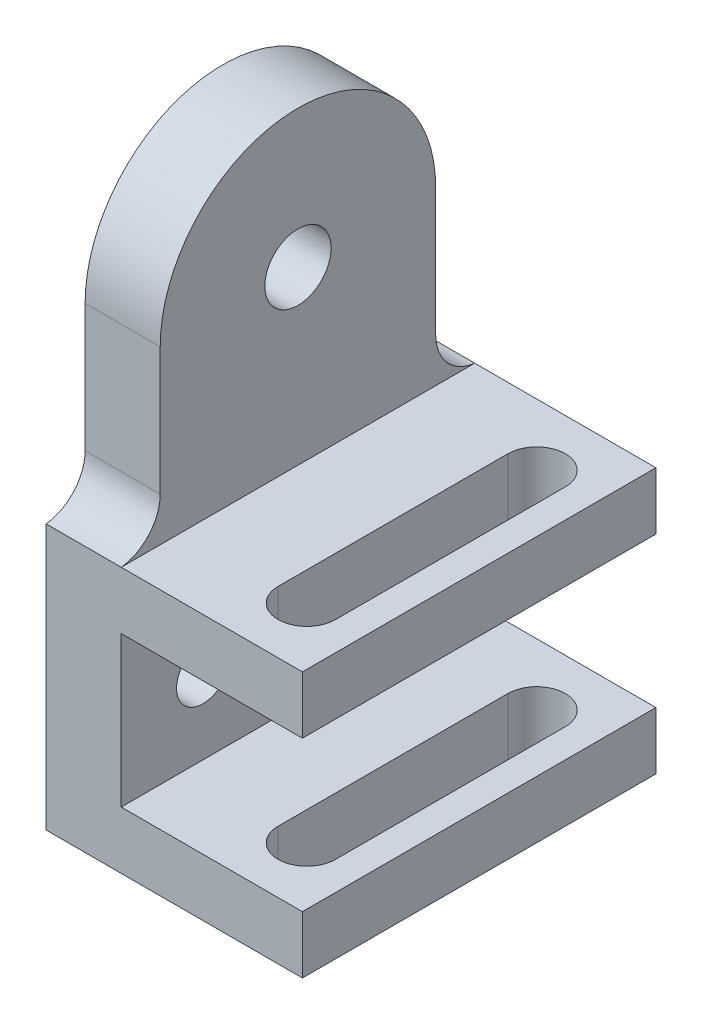
ISO-10303-21;
HEADER;
FILE_DESCRIPTION(('STEP AP214'),'2;1');
FILE_NAME('part.step','',(''),(''),'','','');
FILE_SCHEMA(('AUTOMOTIVE_DESIGN { 1 0 10303 214 1 1 1 1 }'));
ENDSEC;
DATA;
#1=APPLICATION_CONTEXT('core data for automotive mechanical design processes');
#2=APPLICATION_PROTOCOL_DEFINITION('international standard','automotive_design',2000,#1);
#3=PRODUCT_CONTEXT('',#1,'mechanical');
#4=PRODUCT('Part','Part','',(#3));
#5=PRODUCT_RELATED_PRODUCT_CATEGORY('part','',(#4));
#6=PRODUCT_DEFINITION_FORMATION('','',#4);
#7=PRODUCT_DEFINITION_CONTEXT('part definition',#1,'design');
#8=PRODUCT_DEFINITION('design','',#6,#7);
#9=PRODUCT_DEFINITION_SHAPE('','',#8);
#10=(LENGTH_UNIT() NAMED_UNIT(*) SI_UNIT(.MILLI.,.METRE.));
#11=(NAMED_UNIT(*) PLANE_ANGLE_UNIT() SI_UNIT($,.RADIAN.));
#12=(NAMED_UNIT(*) SI_UNIT($,.STERADIAN.) SOLID_ANGLE_UNIT());
#13=UNCERTAINTY_MEASURE_WITH_UNIT(LENGTH_MEASURE(1.E-05),#10,'distance_accuracy_value','');
#14=(GEOMETRIC_REPRESENTATION_CONTEXT(3) GLOBAL_UNCERTAINTY_ASSIGNED_CONTEXT((#13)) GLOBAL_UNIT_ASSIGNED_CONTEXT((#10,
#11,#12)) REPRESENTATION_CONTEXT('',''));
#15=CARTESIAN_POINT('',(0.,0.,0.));
#16=DIRECTION('',(0.,0.,1.));
#17=DIRECTION('',(1.,0.,0.));
#18=AXIS2_PLACEMENT_3D('',#15,#16,#17);
#19=CARTESIAN_POINT('',(0.,0.,40.));
#20=DIRECTION('',(1.,0.,0.));
#21=DIRECTION('',(0.,0.,-1.));
#22=AXIS2_PLACEMENT_3D('',#19,#20,#21);
#23=PLANE('',#22);
#24=CARTESIAN_POINT('',(0.,30.,-21.5));
#25=DIRECTION('',(1.,0.,0.));
#26=DIRECTION('',(0.,0.,-1.));
#27=AXIS2_PLACEMENT_3D('',#24,#25,#26);
#28=CIRCLE('',#27,6.);
#29=CARTESIAN_POINT('',(0.,30.,-27.5));
#30=VERTEX_POINT('',#29);
#31=EDGE_CURVE('E259',#30,#30,#28,.T.);
#32=ORIENTED_EDGE('',*,*,#31,.T.);
#33=EDGE_LOOP('',(#32));
#34=FACE_BOUND('',#33,.T.);
#35=CARTESIAN_POINT('',(0.,30.,21.5));
#36=DIRECTION('',(1.,0.,0.));
#37=DIRECTION('',(0.,0.,-1.));
#38=AXIS2_PLACEMENT_3D('',#35,#36,#37);
#39=CIRCLE('',#38,6.);
#40=CARTESIAN_POINT('',(0.,30.,15.5));
#41=VERTEX_POINT('',#40);
#42=EDGE_CURVE('E255',#41,#41,#39,.T.);
#43=ORIENTED_EDGE('',*,*,#42,.T.);
#44=EDGE_LOOP('',(#43));
#45=FACE_BOUND('',#44,.T.);
#46=CARTESIAN_POINT('',(0.,98.8253035818014,0.));
#47=DIRECTION('',(1.,0.,0.));
#48=DIRECTION('',(0.,0.,-1.));
#49=AXIS2_PLACEMENT_3D('',#46,#47,#48);
#50=CIRCLE('',#49,7.5);
#51=CARTESIAN_POINT('',(0.,98.8253035818014,-7.5));
#52=VERTEX_POINT('',#51);
#53=EDGE_CURVE('E264',#52,#52,#50,.T.);
#54=ORIENTED_EDGE('',*,*,#53,.T.);
#55=EDGE_LOOP('',(#54));
#56=FACE_BOUND('',#55,.T.);
#57=DIRECTION('',(0.,-1.,0.));
#58=VECTOR('',#57,1.);
#59=CARTESIAN_POINT('',(0.,0.,31.1746964181986));
#60=LINE('',#59,#58);
#61=CARTESIAN_POINT('',(0.,98.8253035818014,31.1746964181986));
#62=VERTEX_POINT('',#61);
#63=CARTESIAN_POINT('',(0.,69.9307647401936,31.1746964181986));
#64=VERTEX_POINT('',#63);
#65=EDGE_CURVE('E285',#62,#64,#60,.T.);
#66=ORIENTED_EDGE('',*,*,#65,.F.);
#67=CARTESIAN_POINT('',(0.,98.8253035818014,0.));
#68=DIRECTION('',(1.,0.,0.));
#69=DIRECTION('',(0.,0.,-1.));
#70=AXIS2_PLACEMENT_3D('',#67,#68,#69);
#71=CIRCLE('',#70,31.1746964181986);
#72=CARTESIAN_POINT('',(0.,98.8253035818014,-31.1746964181986));
#73=VERTEX_POINT('',#72);
#74=EDGE_CURVE('E297',#73,#62,#71,.T.);
#75=ORIENTED_EDGE('',*,*,#74,.F.);
#76=DIRECTION('',(0.,1.,0.));
#77=VECTOR('',#76,1.);
#78=CARTESIAN_POINT('',(0.,0.,-31.1746964181986));
#79=LINE('',#78,#77);
#80=CARTESIAN_POINT('',(0.,69.9307647401936,-31.1746964181986));
#81=VERTEX_POINT('',#80);
#82=EDGE_CURVE('E299',#81,#73,#79,.T.);
#83=ORIENTED_EDGE('',*,*,#82,.F.);
#84=CARTESIAN_POINT('',(0.,69.9307647401936,-41.1746964181986));
#85=DIRECTION('',(1.,0.,0.));
#86=DIRECTION('',(0.,0.,-1.));
#87=AXIS2_PLACEMENT_3D('',#84,#85,#86);
#88=CIRCLE('',#87,10.);
#89=CARTESIAN_POINT('',(0.,60.,-40.));
#90=VERTEX_POINT('',#89);
#91=EDGE_CURVE('E293',#90,#81,#88,.F.);
#92=ORIENTED_EDGE('',*,*,#91,.F.);
#93=DIRECTION('',(0.,-1.,0.));
#94=VECTOR('',#93,1.);
#95=CARTESIAN_POINT('',(0.,0.,-40.));
#96=LINE('',#95,#94);
#97=CARTESIAN_POINT('',(0.,0.,-40.));
#98=VERTEX_POINT('',#97);
#99=EDGE_CURVE('E304',#90,#98,#96,.T.);
#100=ORIENTED_EDGE('',*,*,#99,.T.);
#101=DIRECTION('',(0.,0.,-1.));
#102=VECTOR('',#101,1.);
#103=CARTESIAN_POINT('',(0.,0.,40.));
#104=LINE('',#103,#102);
#105=CARTESIAN_POINT('',(0.,0.,40.));
#106=VERTEX_POINT('',#105);
#107=EDGE_CURVE('E359',#106,#98,#104,.T.);
#108=ORIENTED_EDGE('',*,*,#107,.F.);
#109=DIRECTION('',(0.,-1.,0.));
#110=VECTOR('',#109,1.);
#111=CARTESIAN_POINT('',(0.,0.,40.));
#112=LINE('',#111,#110);
#113=CARTESIAN_POINT('',(0.,60.,40.));
#114=VERTEX_POINT('',#113);
#115=EDGE_CURVE('E305',#114,#106,#112,.T.);
#116=ORIENTED_EDGE('',*,*,#115,.F.);
#117=CARTESIAN_POINT('',(0.,69.9307647401936,41.1746964181986));
#118=DIRECTION('',(1.,0.,0.));
#119=DIRECTION('',(0.,0.,-1.));
#120=AXIS2_PLACEMENT_3D('',#117,#118,#119);
#121=CIRCLE('',#120,10.);
#122=EDGE_CURVE('E279',#114,#64,#121,.T.);
#123=ORIENTED_EDGE('',*,*,#122,.T.);
#124=EDGE_LOOP('',(#66,#75,#83,#92,#100,#108,#116,#123));
#125=FACE_BOUND('',#124,.T.);
#126=ADVANCED_FACE('F39',(#34,#45,#56,#125),#23,.F.);
#127=CARTESIAN_POINT('',(17.,60.,40.));
#128=DIRECTION('',(-1.,0.,0.));
#129=DIRECTION('',(0.,0.,1.));
#130=AXIS2_PLACEMENT_3D('',#127,#128,#129);
#131=PLANE('',#130);
#132=CARTESIAN_POINT('',(17.,98.8253035818014,0.));
#133=DIRECTION('',(1.,0.,0.));
#134=DIRECTION('',(0.,0.,-1.));
#135=AXIS2_PLACEMENT_3D('',#132,#133,#134);
#136=CIRCLE('',#135,7.5);
#137=CARTESIAN_POINT('',(17.,98.8253035818014,-7.5));
#138=VERTEX_POINT('',#137);
#139=EDGE_CURVE('E265',#138,#138,#136,.T.);
#140=ORIENTED_EDGE('',*,*,#139,.F.);
#141=EDGE_LOOP('',(#140));
#142=FACE_BOUND('',#141,.T.);
#143=CARTESIAN_POINT('',(17.,98.8253035818014,0.));
#144=DIRECTION('',(1.,0.,0.));
#145=DIRECTION('',(0.,0.,-1.));
#146=AXIS2_PLACEMENT_3D('',#143,#144,#145);
#147=CIRCLE('',#146,31.1746964181986);
#148=CARTESIAN_POINT('',(17.,98.8253035818014,-31.1746964181986));
#149=VERTEX_POINT('',#148);
#150=CARTESIAN_POINT('',(17.,98.8253035818014,31.1746964181986));
#151=VERTEX_POINT('',#150);
#152=EDGE_CURVE('E289',#149,#151,#147,.T.);
#153=ORIENTED_EDGE('',*,*,#152,.T.);
#154=DIRECTION('',(0.,-1.,0.));
#155=VECTOR('',#154,1.);
#156=CARTESIAN_POINT('',(17.,0.,31.1746964181986));
#157=LINE('',#156,#155);
#158=CARTESIAN_POINT('',(17.,69.9307647401936,31.1746964181986));
#159=VERTEX_POINT('',#158);
#160=EDGE_CURVE('E271',#151,#159,#157,.T.);
#161=ORIENTED_EDGE('',*,*,#160,.T.);
#162=CARTESIAN_POINT('',(17.,69.9307647401936,41.1746964181986));
#163=DIRECTION('',(1.,0.,0.));
#164=DIRECTION('',(0.,0.,-1.));
#165=AXIS2_PLACEMENT_3D('',#162,#163,#164);
#166=CIRCLE('',#165,10.);
#167=CARTESIAN_POINT('',(17.,60.,40.));
#168=VERTEX_POINT('',#167);
#169=EDGE_CURVE('E268',#168,#159,#166,.T.);
#170=ORIENTED_EDGE('',*,*,#169,.F.);
#171=DIRECTION('',(0.,0.,-1.));
#172=VECTOR('',#171,1.);
#173=CARTESIAN_POINT('',(17.,60.,40.));
#174=LINE('',#173,#172);
#175=CARTESIAN_POINT('',(17.,60.,-40.));
#176=VERTEX_POINT('',#175);
#177=EDGE_CURVE('E321',#168,#176,#174,.T.);
#178=ORIENTED_EDGE('',*,*,#177,.T.);
#179=CARTESIAN_POINT('',(17.,69.9307647401936,-41.1746964181986));
#180=DIRECTION('',(1.,0.,0.));
#181=DIRECTION('',(0.,0.,-1.));
#182=AXIS2_PLACEMENT_3D('',#179,#180,#181);
#183=CIRCLE('',#182,10.);
#184=CARTESIAN_POINT('',(17.,69.9307647401936,-31.1746964181986));
#185=VERTEX_POINT('',#184);
#186=EDGE_CURVE('E283',#176,#185,#183,.F.);
#187=ORIENTED_EDGE('',*,*,#186,.T.);
#188=DIRECTION('',(0.,1.,0.));
#189=VECTOR('',#188,1.);
#190=CARTESIAN_POINT('',(17.,0.,-31.1746964181986));
#191=LINE('',#190,#189);
#192=EDGE_CURVE('E286',#185,#149,#191,.T.);
#193=ORIENTED_EDGE('',*,*,#192,.T.);
#194=EDGE_LOOP('',(#153,#161,#170,#178,#187,#193));
#195=FACE_BOUND('',#194,.T.);
#196=ADVANCED_FACE('F373',(#142,#195),#131,.F.);
#197=CARTESIAN_POINT('',(0.,0.,-40.));
#198=DIRECTION('',(0.,0.,-1.));
#199=DIRECTION('',(-1.,0.,0.));
#200=AXIS2_PLACEMENT_3D('',#197,#198,#199);
#201=PLANE('',#200);
#202=ORIENTED_EDGE('',*,*,#99,.F.);
#203=DIRECTION('',(1.,0.,0.));
#204=VECTOR('',#203,1.);
#205=CARTESIAN_POINT('',(-63.,60.,-40.));
#206=LINE('',#205,#204);
#207=EDGE_CURVE('E46',#90,#176,#206,.T.);
#208=ORIENTED_EDGE('',*,*,#207,.T.);
#209=DIRECTION('',(-1.,0.,0.));
#210=VECTOR('',#209,1.);
#211=CARTESIAN_POINT('',(58.,60.,-40.));
#212=LINE('',#211,#210);
#213=CARTESIAN_POINT('',(58.,60.,-40.));
#214=VERTEX_POINT('',#213);
#215=EDGE_CURVE('E308',#214,#176,#212,.T.);
#216=ORIENTED_EDGE('',*,*,#215,.F.);
#217=DIRECTION('',(0.,1.,0.));
#218=VECTOR('',#217,1.);
#219=CARTESIAN_POINT('',(58.,47.,-40.));
#220=LINE('',#219,#218);
#221=CARTESIAN_POINT('',(58.,47.,-40.));
#222=VERTEX_POINT('',#221);
#223=EDGE_CURVE('E334',#222,#214,#220,.T.);
#224=ORIENTED_EDGE('',*,*,#223,.F.);
#225=DIRECTION('',(1.,0.,0.));
#226=VECTOR('',#225,1.);
#227=CARTESIAN_POINT('',(17.,47.,-40.));
#228=LINE('',#227,#226);
#229=CARTESIAN_POINT('',(17.,47.,-40.));
#230=VERTEX_POINT('',#229);
#231=EDGE_CURVE('E332',#230,#222,#228,.T.);
#232=ORIENTED_EDGE('',*,*,#231,.F.);
#233=DIRECTION('',(0.,1.,0.));
#234=VECTOR('',#233,1.);
#235=CARTESIAN_POINT('',(17.,13.,-40.));
#236=LINE('',#235,#234);
#237=CARTESIAN_POINT('',(17.,13.,-40.));
#238=VERTEX_POINT('',#237);
#239=EDGE_CURVE('E328',#238,#230,#236,.T.);
#240=ORIENTED_EDGE('',*,*,#239,.F.);
#241=DIRECTION('',(-1.,0.,0.));
#242=VECTOR('',#241,1.);
#243=CARTESIAN_POINT('',(58.,13.,-40.));
#244=LINE('',#243,#242);
#245=CARTESIAN_POINT('',(58.,13.,-40.));
#246=VERTEX_POINT('',#245);
#247=EDGE_CURVE('E330',#246,#238,#244,.T.);
#248=ORIENTED_EDGE('',*,*,#247,.F.);
#249=DIRECTION('',(0.,1.,0.));
#250=VECTOR('',#249,1.);
#251=CARTESIAN_POINT('',(58.,0.,-40.));
#252=LINE('',#251,#250);
#253=CARTESIAN_POINT('',(58.,0.,-40.));
#254=VERTEX_POINT('',#253);
#255=EDGE_CURVE('E324',#254,#246,#252,.T.);
#256=ORIENTED_EDGE('',*,*,#255,.F.);
#257=DIRECTION('',(1.,0.,0.));
#258=VECTOR('',#257,1.);
#259=CARTESIAN_POINT('',(0.,0.,-40.));
#260=LINE('',#259,#258);
#261=EDGE_CURVE('E323',#98,#254,#260,.T.);
#262=ORIENTED_EDGE('',*,*,#261,.F.);
#263=EDGE_LOOP('',(#202,#208,#216,#224,#232,#240,#248,#256,#262));
#264=FACE_BOUND('',#263,.T.);
#265=ADVANCED_FACE('F361',(#264),#201,.T.);
#266=CARTESIAN_POINT('',(0.,0.,40.));
#267=DIRECTION('',(0.,1.,0.));
#268=DIRECTION('',(0.,0.,1.));
#269=AXIS2_PLACEMENT_3D('',#266,#267,#268);
#270=PLANE('',#269);
#271=DIRECTION('',(0.,0.,1.));
#272=VECTOR('',#271,1.);
#273=CARTESIAN_POINT('',(38.5,0.,40.));
#274=LINE('',#273,#272);
#275=CARTESIAN_POINT('',(38.5,0.,-26.));
#276=VERTEX_POINT('',#275);
#277=CARTESIAN_POINT('',(38.5,0.,26.));
#278=VERTEX_POINT('',#277);
#279=EDGE_CURVE('E236',#276,#278,#274,.T.);
#280=ORIENTED_EDGE('',*,*,#279,.T.);
#281=CARTESIAN_POINT('',(45.,0.,26.));
#282=DIRECTION('',(0.,1.,0.));
#283=DIRECTION('',(0.,0.,1.));
#284=AXIS2_PLACEMENT_3D('',#281,#282,#283);
#285=CIRCLE('',#284,6.5);
#286=CARTESIAN_POINT('',(51.5,0.,26.));
#287=VERTEX_POINT('',#286);
#288=EDGE_CURVE('E249',#278,#287,#285,.T.);
#289=ORIENTED_EDGE('',*,*,#288,.T.);
#290=DIRECTION('',(0.,0.,-1.));
#291=VECTOR('',#290,1.);
#292=CARTESIAN_POINT('',(51.5,0.,40.));
#293=LINE('',#292,#291);
#294=CARTESIAN_POINT('',(51.5,0.,-26.));
#295=VERTEX_POINT('',#294);
#296=EDGE_CURVE('E225',#287,#295,#293,.T.);
#297=ORIENTED_EDGE('',*,*,#296,.T.);
#298=CARTESIAN_POINT('',(45.,0.,-26.));
#299=DIRECTION('',(0.,1.,0.));
#300=DIRECTION('',(0.,0.,1.));
#301=AXIS2_PLACEMENT_3D('',#298,#299,#300);
#302=CIRCLE('',#301,6.5);
#303=EDGE_CURVE('E228',#295,#276,#302,.T.);
#304=ORIENTED_EDGE('',*,*,#303,.T.);
#305=EDGE_LOOP('',(#280,#289,#297,#304));
#306=FACE_BOUND('',#305,.T.);
#307=ORIENTED_EDGE('',*,*,#261,.T.);
#308=DIRECTION('',(0.,0.,-1.));
#309=VECTOR('',#308,1.);
#310=CARTESIAN_POINT('',(58.,0.,40.));
#311=LINE('',#310,#309);
#312=CARTESIAN_POINT('',(58.,0.,40.));
#313=VERTEX_POINT('',#312);
#314=EDGE_CURVE('E353',#313,#254,#311,.T.);
#315=ORIENTED_EDGE('',*,*,#314,.F.);
#316=DIRECTION('',(1.,0.,0.));
#317=VECTOR('',#316,1.);
#318=CARTESIAN_POINT('',(0.,0.,40.));
#319=LINE('',#318,#317);
#320=EDGE_CURVE('E303',#106,#313,#319,.T.);
#321=ORIENTED_EDGE('',*,*,#320,.F.);
#322=ORIENTED_EDGE('',*,*,#107,.T.);
#323=EDGE_LOOP('',(#307,#315,#321,#322));
#324=FACE_BOUND('',#323,.T.);
#325=ADVANCED_FACE('F406',(#306,#324),#270,.F.);
#326=CARTESIAN_POINT('',(58.,0.,40.));
#327=DIRECTION('',(-1.,0.,0.));
#328=DIRECTION('',(0.,0.,1.));
#329=AXIS2_PLACEMENT_3D('',#326,#327,#328);
#330=PLANE('',#329);
#331=ORIENTED_EDGE('',*,*,#255,.T.);
#332=DIRECTION('',(0.,0.,-1.));
#333=VECTOR('',#332,1.);
#334=CARTESIAN_POINT('',(58.,13.,40.));
#335=LINE('',#334,#333);
#336=CARTESIAN_POINT('',(58.,13.,40.));
#337=VERTEX_POINT('',#336);
#338=EDGE_CURVE('E351',#337,#246,#335,.T.);
#339=ORIENTED_EDGE('',*,*,#338,.F.);
#340=DIRECTION('',(0.,1.,0.));
#341=VECTOR('',#340,1.);
#342=CARTESIAN_POINT('',(58.,0.,40.));
#343=LINE('',#342,#341);
#344=EDGE_CURVE('E306',#313,#337,#343,.T.);
#345=ORIENTED_EDGE('',*,*,#344,.F.);
#346=ORIENTED_EDGE('',*,*,#314,.T.);
#347=EDGE_LOOP('',(#331,#339,#345,#346));
#348=FACE_BOUND('',#347,.T.);
#349=ADVANCED_FACE('F402',(#348),#330,.F.);
#350=CARTESIAN_POINT('',(58.,13.,40.));
#351=DIRECTION('',(0.,-1.,0.));
#352=DIRECTION('',(0.,0.,-1.));
#353=AXIS2_PLACEMENT_3D('',#350,#351,#352);
#354=PLANE('',#353);
#355=DIRECTION('',(0.,0.,1.));
#356=VECTOR('',#355,1.);
#357=CARTESIAN_POINT('',(51.5,13.,40.));
#358=LINE('',#357,#356);
#359=CARTESIAN_POINT('',(51.5,13.,-26.));
#360=VERTEX_POINT('',#359);
#361=CARTESIAN_POINT('',(51.5,13.,26.));
#362=VERTEX_POINT('',#361);
#363=EDGE_CURVE('E218',#360,#362,#358,.T.);
#364=ORIENTED_EDGE('',*,*,#363,.T.);
#365=CARTESIAN_POINT('',(45.,13.,26.));
#366=DIRECTION('',(0.,-1.,0.));
#367=DIRECTION('',(0.,0.,-1.));
#368=AXIS2_PLACEMENT_3D('',#365,#366,#367);
#369=CIRCLE('',#368,6.5);
#370=CARTESIAN_POINT('',(38.5,13.,26.));
#371=VERTEX_POINT('',#370);
#372=EDGE_CURVE('E243',#362,#371,#369,.T.);
#373=ORIENTED_EDGE('',*,*,#372,.T.);
#374=DIRECTION('',(0.,0.,-1.));
#375=VECTOR('',#374,1.);
#376=CARTESIAN_POINT('',(38.5,13.,40.));
#377=LINE('',#376,#375);
#378=CARTESIAN_POINT('',(38.5,13.,-26.));
#379=VERTEX_POINT('',#378);
#380=EDGE_CURVE('E233',#371,#379,#377,.T.);
#381=ORIENTED_EDGE('',*,*,#380,.T.);
#382=CARTESIAN_POINT('',(45.,13.,-26.));
#383=DIRECTION('',(0.,-1.,0.));
#384=DIRECTION('',(0.,0.,-1.));
#385=AXIS2_PLACEMENT_3D('',#382,#383,#384);
#386=CIRCLE('',#385,6.5);
#387=EDGE_CURVE('E226',#379,#360,#386,.T.);
#388=ORIENTED_EDGE('',*,*,#387,.T.);
#389=EDGE_LOOP('',(#364,#373,#381,#388));
#390=FACE_BOUND('',#389,.T.);
#391=ORIENTED_EDGE('',*,*,#247,.T.);
#392=DIRECTION('',(0.,0.,-1.));
#393=VECTOR('',#392,1.);
#394=CARTESIAN_POINT('',(17.,13.,40.));
#395=LINE('',#394,#393);
#396=CARTESIAN_POINT('',(17.,13.,40.));
#397=VERTEX_POINT('',#396);
#398=EDGE_CURVE('E346',#397,#238,#395,.T.);
#399=ORIENTED_EDGE('',*,*,#398,.F.);
#400=DIRECTION('',(-1.,0.,0.));
#401=VECTOR('',#400,1.);
#402=CARTESIAN_POINT('',(58.,13.,40.));
#403=LINE('',#402,#401);
#404=EDGE_CURVE('E309',#337,#397,#403,.T.);
#405=ORIENTED_EDGE('',*,*,#404,.F.);
#406=ORIENTED_EDGE('',*,*,#338,.T.);
#407=EDGE_LOOP('',(#391,#399,#405,#406));
#408=FACE_BOUND('',#407,.T.);
#409=ADVANCED_FACE('F399',(#390,#408),#354,.F.);
#410=CARTESIAN_POINT('',(17.,13.,40.));
#411=DIRECTION('',(-1.,0.,0.));
#412=DIRECTION('',(0.,0.,1.));
#413=AXIS2_PLACEMENT_3D('',#410,#411,#412);
#414=PLANE('',#413);
#415=CARTESIAN_POINT('',(17.,30.,-21.5));
#416=DIRECTION('',(1.,0.,0.));
#417=DIRECTION('',(0.,0.,1.));
#418=AXIS2_PLACEMENT_3D('',#415,#416,#417);
#419=CIRCLE('',#418,6.);
#420=CARTESIAN_POINT('',(17.,30.,-15.5));
#421=VERTEX_POINT('',#420);
#422=EDGE_CURVE('E253',#421,#421,#419,.T.);
#423=ORIENTED_EDGE('',*,*,#422,.F.);
#424=EDGE_LOOP('',(#423));
#425=FACE_BOUND('',#424,.T.);
#426=CARTESIAN_POINT('',(17.,30.,21.5));
#427=DIRECTION('',(1.,0.,0.));
#428=DIRECTION('',(0.,0.,-1.));
#429=AXIS2_PLACEMENT_3D('',#426,#427,#428);
#430=CIRCLE('',#429,6.);
#431=CARTESIAN_POINT('',(17.,30.,15.5));
#432=VERTEX_POINT('',#431);
#433=EDGE_CURVE('E248',#432,#432,#430,.T.);
#434=ORIENTED_EDGE('',*,*,#433,.F.);
#435=EDGE_LOOP('',(#434));
#436=FACE_BOUND('',#435,.T.);
#437=ORIENTED_EDGE('',*,*,#239,.T.);
#438=DIRECTION('',(0.,0.,-1.));
#439=VECTOR('',#438,1.);
#440=CARTESIAN_POINT('',(17.,47.,40.));
#441=LINE('',#440,#439);
#442=CARTESIAN_POINT('',(17.,47.,40.));
#443=VERTEX_POINT('',#442);
#444=EDGE_CURVE('E343',#443,#230,#441,.T.);
#445=ORIENTED_EDGE('',*,*,#444,.F.);
#446=DIRECTION('',(0.,1.,0.));
#447=VECTOR('',#446,1.);
#448=CARTESIAN_POINT('',(17.,13.,40.));
#449=LINE('',#448,#447);
#450=EDGE_CURVE('E315',#397,#443,#449,.T.);
#451=ORIENTED_EDGE('',*,*,#450,.F.);
#452=ORIENTED_EDGE('',*,*,#398,.T.);
#453=EDGE_LOOP('',(#437,#445,#451,#452));
#454=FACE_BOUND('',#453,.T.);
#455=ADVANCED_FACE('F392',(#425,#436,#454),#414,.F.);
#456=CARTESIAN_POINT('',(17.,47.,40.));
#457=DIRECTION('',(0.,1.,0.));
#458=DIRECTION('',(0.,0.,1.));
#459=AXIS2_PLACEMENT_3D('',#456,#457,#458);
#460=PLANE('',#459);
#461=DIRECTION('',(0.,0.,1.));
#462=VECTOR('',#461,1.);
#463=CARTESIAN_POINT('',(38.5,47.,40.));
#464=LINE('',#463,#462);
#465=CARTESIAN_POINT('',(38.5,47.,-26.));
#466=VERTEX_POINT('',#465);
#467=CARTESIAN_POINT('',(38.5,47.,26.));
#468=VERTEX_POINT('',#467);
#469=EDGE_CURVE('E234',#466,#468,#464,.T.);
#470=ORIENTED_EDGE('',*,*,#469,.T.);
#471=CARTESIAN_POINT('',(45.,47.,26.));
#472=DIRECTION('',(0.,1.,0.));
#473=DIRECTION('',(0.,0.,1.));
#474=AXIS2_PLACEMENT_3D('',#471,#472,#473);
#475=CIRCLE('',#474,6.5);
#476=CARTESIAN_POINT('',(51.5,47.,26.));
#477=VERTEX_POINT('',#476);
#478=EDGE_CURVE('E241',#468,#477,#475,.T.);
#479=ORIENTED_EDGE('',*,*,#478,.T.);
#480=DIRECTION('',(0.,0.,-1.));
#481=VECTOR('',#480,1.);
#482=CARTESIAN_POINT('',(51.5,47.,40.));
#483=LINE('',#482,#481);
#484=CARTESIAN_POINT('',(51.5,47.,-26.));
#485=VERTEX_POINT('',#484);
#486=EDGE_CURVE('E220',#477,#485,#483,.T.);
#487=ORIENTED_EDGE('',*,*,#486,.T.);
#488=CARTESIAN_POINT('',(45.,47.,-26.));
#489=DIRECTION('',(0.,1.,0.));
#490=DIRECTION('',(0.,0.,1.));
#491=AXIS2_PLACEMENT_3D('',#488,#489,#490);
#492=CIRCLE('',#491,6.5);
#493=EDGE_CURVE('E187',#485,#466,#492,.T.);
#494=ORIENTED_EDGE('',*,*,#493,.T.);
#495=EDGE_LOOP('',(#470,#479,#487,#494));
#496=FACE_BOUND('',#495,.T.);
#497=ORIENTED_EDGE('',*,*,#231,.T.);
#498=DIRECTION('',(0.,0.,-1.));
#499=VECTOR('',#498,1.);
#500=CARTESIAN_POINT('',(58.,47.,40.));
#501=LINE('',#500,#499);
#502=CARTESIAN_POINT('',(58.,47.,40.));
#503=VERTEX_POINT('',#502);
#504=EDGE_CURVE('E344',#503,#222,#501,.T.);
#505=ORIENTED_EDGE('',*,*,#504,.F.);
#506=DIRECTION('',(1.,0.,0.));
#507=VECTOR('',#506,1.);
#508=CARTESIAN_POINT('',(17.,47.,40.));
#509=LINE('',#508,#507);
#510=EDGE_CURVE('E314',#443,#503,#509,.T.);
#511=ORIENTED_EDGE('',*,*,#510,.F.);
#512=ORIENTED_EDGE('',*,*,#444,.T.);
#513=EDGE_LOOP('',(#497,#505,#511,#512));
#514=FACE_BOUND('',#513,.T.);
#515=ADVANCED_FACE('F386',(#496,#514),#460,.F.);
#516=CARTESIAN_POINT('',(58.,47.,40.));
#517=DIRECTION('',(-1.,0.,0.));
#518=DIRECTION('',(0.,0.,1.));
#519=AXIS2_PLACEMENT_3D('',#516,#517,#518);
#520=PLANE('',#519);
#521=ORIENTED_EDGE('',*,*,#223,.T.);
#522=DIRECTION('',(0.,0.,-1.));
#523=VECTOR('',#522,1.);
#524=CARTESIAN_POINT('',(58.,60.,40.));
#525=LINE('',#524,#523);
#526=CARTESIAN_POINT('',(58.,60.,40.));
#527=VERTEX_POINT('',#526);
#528=EDGE_CURVE('E338',#527,#214,#525,.T.);
#529=ORIENTED_EDGE('',*,*,#528,.F.);
#530=DIRECTION('',(0.,1.,0.));
#531=VECTOR('',#530,1.);
#532=CARTESIAN_POINT('',(58.,47.,40.));
#533=LINE('',#532,#531);
#534=EDGE_CURVE('E316',#503,#527,#533,.T.);
#535=ORIENTED_EDGE('',*,*,#534,.F.);
#536=ORIENTED_EDGE('',*,*,#504,.T.);
#537=EDGE_LOOP('',(#521,#529,#535,#536));
#538=FACE_BOUND('',#537,.T.);
#539=ADVANCED_FACE('F383',(#538),#520,.F.);
#540=CARTESIAN_POINT('',(58.,60.,40.));
#541=DIRECTION('',(0.,-1.,0.));
#542=DIRECTION('',(0.,0.,-1.));
#543=AXIS2_PLACEMENT_3D('',#540,#541,#542);
#544=PLANE('',#543);
#545=DIRECTION('',(0.,0.,-1.));
#546=VECTOR('',#545,1.);
#547=CARTESIAN_POINT('',(51.5,60.,26.));
#548=LINE('',#547,#546);
#549=CARTESIAN_POINT('',(51.5,60.,26.));
#550=VERTEX_POINT('',#549);
#551=CARTESIAN_POINT('',(51.5,60.,-26.));
#552=VERTEX_POINT('',#551);
#553=EDGE_CURVE('E191',#550,#552,#548,.T.);
#554=ORIENTED_EDGE('',*,*,#553,.F.);
#555=CARTESIAN_POINT('',(45.,60.,26.));
#556=DIRECTION('',(0.,1.,0.));
#557=DIRECTION('',(0.,0.,1.));
#558=AXIS2_PLACEMENT_3D('',#555,#556,#557);
#559=CIRCLE('',#558,6.5);
#560=CARTESIAN_POINT('',(38.5,60.,26.));
#561=VERTEX_POINT('',#560);
#562=EDGE_CURVE('E199',#561,#550,#559,.T.);
#563=ORIENTED_EDGE('',*,*,#562,.F.);
#564=DIRECTION('',(0.,0.,1.));
#565=VECTOR('',#564,1.);
#566=CARTESIAN_POINT('',(38.5,60.,26.));
#567=LINE('',#566,#565);
#568=CARTESIAN_POINT('',(38.5,60.,-26.));
#569=VERTEX_POINT('',#568);
#570=EDGE_CURVE('E202',#569,#561,#567,.T.);
#571=ORIENTED_EDGE('',*,*,#570,.F.);
#572=CARTESIAN_POINT('',(45.,60.,-26.));
#573=DIRECTION('',(0.,1.,0.));
#574=DIRECTION('',(0.,0.,1.));
#575=AXIS2_PLACEMENT_3D('',#572,#573,#574);
#576=CIRCLE('',#575,6.5);
#577=EDGE_CURVE('E183',#552,#569,#576,.T.);
#578=ORIENTED_EDGE('',*,*,#577,.F.);
#579=EDGE_LOOP('',(#554,#563,#571,#578));
#580=FACE_BOUND('',#579,.T.);
#581=ORIENTED_EDGE('',*,*,#215,.T.);
#582=ORIENTED_EDGE('',*,*,#177,.F.);
#583=DIRECTION('',(-1.,0.,0.));
#584=VECTOR('',#583,1.);
#585=CARTESIAN_POINT('',(58.,60.,40.));
#586=LINE('',#585,#584);
#587=EDGE_CURVE('E318',#527,#168,#586,.T.);
#588=ORIENTED_EDGE('',*,*,#587,.F.);
#589=ORIENTED_EDGE('',*,*,#528,.T.);
#590=EDGE_LOOP('',(#581,#582,#588,#589));
#591=FACE_BOUND('',#590,.T.);
#592=ADVANCED_FACE('F205',(#580,#591),#544,.F.);
#593=CARTESIAN_POINT('',(0.,0.,40.));
#594=DIRECTION('',(0.,0.,-1.));
#595=DIRECTION('',(-1.,0.,0.));
#596=AXIS2_PLACEMENT_3D('',#593,#594,#595);
#597=PLANE('',#596);
#598=ORIENTED_EDGE('',*,*,#587,.T.);
#599=DIRECTION('',(1.,0.,0.));
#600=VECTOR('',#599,1.);
#601=CARTESIAN_POINT('',(-63.,60.,40.));
#602=LINE('',#601,#600);
#603=EDGE_CURVE('E11',#168,#114,#602,.F.);
#604=ORIENTED_EDGE('',*,*,#603,.T.);
#605=ORIENTED_EDGE('',*,*,#115,.T.);
#606=ORIENTED_EDGE('',*,*,#320,.T.);
#607=ORIENTED_EDGE('',*,*,#344,.T.);
#608=ORIENTED_EDGE('',*,*,#404,.T.);
#609=ORIENTED_EDGE('',*,*,#450,.T.);
#610=ORIENTED_EDGE('',*,*,#510,.T.);
#611=ORIENTED_EDGE('',*,*,#534,.T.);
#612=EDGE_LOOP('',(#598,#604,#605,#606,#607,#608,#609,#610,#611));
#613=FACE_BOUND('',#612,.T.);
#614=ADVANCED_FACE('F378',(#613),#597,.F.);
#615=CARTESIAN_POINT('',(-63.,0.,-31.1746964181986));
#616=DIRECTION('',(0.,0.,-1.));
#617=DIRECTION('',(0.,1.,0.));
#618=AXIS2_PLACEMENT_3D('',#615,#616,#617);
#619=PLANE('',#618);
#620=ORIENTED_EDGE('',*,*,#82,.T.);
#621=DIRECTION('',(1.,0.,0.));
#622=VECTOR('',#621,1.);
#623=CARTESIAN_POINT('',(-63.,98.8253035818014,-31.1746964181986));
#624=LINE('',#623,#622);
#625=EDGE_CURVE('E295',#73,#149,#624,.T.);
#626=ORIENTED_EDGE('',*,*,#625,.T.);
#627=ORIENTED_EDGE('',*,*,#192,.F.);
#628=DIRECTION('',(1.,0.,0.));
#629=VECTOR('',#628,1.);
#630=CARTESIAN_POINT('',(-63.,69.9307647401936,-31.1746964181986));
#631=LINE('',#630,#629);
#632=EDGE_CURVE('E291',#81,#185,#631,.T.);
#633=ORIENTED_EDGE('',*,*,#632,.F.);
#634=EDGE_LOOP('',(#620,#626,#627,#633));
#635=FACE_BOUND('',#634,.T.);
#636=ADVANCED_FACE('F418',(#635),#619,.T.);
#637=CARTESIAN_POINT('',(-63.,98.8253035818014,0.));
#638=DIRECTION('',(1.,0.,0.));
#639=DIRECTION('',(0.,0.,-1.));
#640=AXIS2_PLACEMENT_3D('',#637,#638,#639);
#641=CYLINDRICAL_SURFACE('',#640,31.1746964181986);
#642=ORIENTED_EDGE('',*,*,#74,.T.);
#643=DIRECTION('',(1.,0.,0.));
#644=VECTOR('',#643,1.);
#645=CARTESIAN_POINT('',(-63.,98.8253035818014,31.1746964181986));
#646=LINE('',#645,#644);
#647=EDGE_CURVE('E274',#62,#151,#646,.T.);
#648=ORIENTED_EDGE('',*,*,#647,.T.);
#649=ORIENTED_EDGE('',*,*,#152,.F.);
#650=ORIENTED_EDGE('',*,*,#625,.F.);
#651=EDGE_LOOP('',(#642,#648,#649,#650));
#652=FACE_BOUND('',#651,.T.);
#653=ADVANCED_FACE('F423',(#652),#641,.T.);
#654=CARTESIAN_POINT('',(-63.,69.9307647401936,-41.1746964181986));
#655=DIRECTION('',(1.,0.,0.));
#656=DIRECTION('',(0.,0.,-1.));
#657=AXIS2_PLACEMENT_3D('',#654,#655,#656);
#658=CYLINDRICAL_SURFACE('',#657,10.);
#659=ORIENTED_EDGE('',*,*,#91,.T.);
#660=ORIENTED_EDGE('',*,*,#632,.T.);
#661=ORIENTED_EDGE('',*,*,#186,.F.);
#662=ORIENTED_EDGE('',*,*,#207,.F.);
#663=EDGE_LOOP('',(#659,#660,#661,#662));
#664=FACE_BOUND('',#663,.T.);
#665=ADVANCED_FACE('F415',(#664),#658,.F.);
#666=CARTESIAN_POINT('',(-63.,0.,31.1746964181986));
#667=DIRECTION('',(0.,0.,1.));
#668=DIRECTION('',(0.,-1.,0.));
#669=AXIS2_PLACEMENT_3D('',#666,#667,#668);
#670=PLANE('',#669);
#671=ORIENTED_EDGE('',*,*,#65,.T.);
#672=DIRECTION('',(1.,0.,0.));
#673=VECTOR('',#672,1.);
#674=CARTESIAN_POINT('',(-63.,69.9307647401936,31.1746964181986));
#675=LINE('',#674,#673);
#676=EDGE_CURVE('E273',#64,#159,#675,.T.);
#677=ORIENTED_EDGE('',*,*,#676,.T.);
#678=ORIENTED_EDGE('',*,*,#160,.F.);
#679=ORIENTED_EDGE('',*,*,#647,.F.);
#680=EDGE_LOOP('',(#671,#677,#678,#679));
#681=FACE_BOUND('',#680,.T.);
#682=ADVANCED_FACE('F421',(#681),#670,.T.);
#683=CARTESIAN_POINT('',(-63.,69.9307647401936,41.1746964181986));
#684=DIRECTION('',(1.,0.,0.));
#685=DIRECTION('',(0.,0.,-1.));
#686=AXIS2_PLACEMENT_3D('',#683,#684,#685);
#687=CYLINDRICAL_SURFACE('',#686,10.);
#688=ORIENTED_EDGE('',*,*,#603,.F.);
#689=ORIENTED_EDGE('',*,*,#169,.T.);
#690=ORIENTED_EDGE('',*,*,#676,.F.);
#691=ORIENTED_EDGE('',*,*,#122,.F.);
#692=EDGE_LOOP('',(#688,#689,#690,#691));
#693=FACE_BOUND('',#692,.T.);
#694=ADVANCED_FACE('F424',(#693),#687,.F.);
#695=CARTESIAN_POINT('',(-63.,98.8253035818014,0.));
#696=DIRECTION('',(1.,0.,0.));
#697=DIRECTION('',(0.,0.,-1.));
#698=AXIS2_PLACEMENT_3D('',#695,#696,#697);
#699=CYLINDRICAL_SURFACE('',#698,7.5);
#700=ORIENTED_EDGE('',*,*,#139,.T.);
#701=EDGE_LOOP('',(#700));
#702=FACE_BOUND('',#701,.T.);
#703=ORIENTED_EDGE('',*,*,#53,.F.);
#704=EDGE_LOOP('',(#703));
#705=FACE_BOUND('',#704,.T.);
#706=ADVANCED_FACE('F426',(#702,#705),#699,.F.);
#707=CARTESIAN_POINT('',(-63.,30.,21.5));
#708=DIRECTION('',(1.,0.,0.));
#709=DIRECTION('',(0.,0.,-1.));
#710=AXIS2_PLACEMENT_3D('',#707,#708,#709);
#711=CYLINDRICAL_SURFACE('',#710,6.);
#712=ORIENTED_EDGE('',*,*,#433,.T.);
#713=EDGE_LOOP('',(#712));
#714=FACE_BOUND('',#713,.T.);
#715=ORIENTED_EDGE('',*,*,#42,.F.);
#716=EDGE_LOOP('',(#715));
#717=FACE_BOUND('',#716,.T.);
#718=ADVANCED_FACE('F433',(#714,#717),#711,.F.);
#719=CARTESIAN_POINT('',(-63.,30.,-21.5));
#720=DIRECTION('',(1.,0.,0.));
#721=DIRECTION('',(0.,0.,-1.));
#722=AXIS2_PLACEMENT_3D('',#719,#720,#721);
#723=CYLINDRICAL_SURFACE('',#722,6.);
#724=ORIENTED_EDGE('',*,*,#422,.T.);
#725=EDGE_LOOP('',(#724));
#726=FACE_BOUND('',#725,.T.);
#727=ORIENTED_EDGE('',*,*,#31,.F.);
#728=EDGE_LOOP('',(#727));
#729=FACE_BOUND('',#728,.T.);
#730=ADVANCED_FACE('F455',(#726,#729),#723,.F.);
#731=CARTESIAN_POINT('',(51.5,-20.,26.));
#732=DIRECTION('',(1.,0.,0.));
#733=DIRECTION('',(0.,0.,-1.));
#734=AXIS2_PLACEMENT_3D('',#731,#732,#733);
#735=PLANE('',#734);
#736=DIRECTION('',(0.,1.,0.));
#737=VECTOR('',#736,1.);
#738=CARTESIAN_POINT('',(51.5,-20.,26.));
#739=LINE('',#738,#737);
#740=EDGE_CURVE('E197',#477,#550,#739,.T.);
#741=ORIENTED_EDGE('',*,*,#740,.T.);
#742=ORIENTED_EDGE('',*,*,#553,.T.);
#743=DIRECTION('',(0.,1.,0.));
#744=VECTOR('',#743,1.);
#745=CARTESIAN_POINT('',(51.5,-20.,-26.));
#746=LINE('',#745,#744);
#747=EDGE_CURVE('E178',#485,#552,#746,.T.);
#748=ORIENTED_EDGE('',*,*,#747,.F.);
#749=ORIENTED_EDGE('',*,*,#486,.F.);
#750=EDGE_LOOP('',(#741,#742,#748,#749));
#751=FACE_BOUND('',#750,.T.);
#752=ADVANCED_FACE('F193',(#751),#735,.F.);
#753=CARTESIAN_POINT('',(45.,-20.,-26.));
#754=DIRECTION('',(0.,1.,0.));
#755=DIRECTION('',(0.,0.,1.));
#756=AXIS2_PLACEMENT_3D('',#753,#754,#755);
#757=CYLINDRICAL_SURFACE('',#756,6.5);
#758=ORIENTED_EDGE('',*,*,#747,.T.);
#759=ORIENTED_EDGE('',*,*,#577,.T.);
#760=DIRECTION('',(0.,1.,0.));
#761=VECTOR('',#760,1.);
#762=CARTESIAN_POINT('',(38.5,-20.,-26.));
#763=LINE('',#762,#761);
#764=EDGE_CURVE('E212',#466,#569,#763,.T.);
#765=ORIENTED_EDGE('',*,*,#764,.F.);
#766=ORIENTED_EDGE('',*,*,#493,.F.);
#767=EDGE_LOOP('',(#758,#759,#765,#766));
#768=FACE_BOUND('',#767,.T.);
#769=ADVANCED_FACE('F185',(#768),#757,.F.);
#770=CARTESIAN_POINT('',(38.5,-20.,26.));
#771=DIRECTION('',(-1.,0.,0.));
#772=DIRECTION('',(0.,0.,1.));
#773=AXIS2_PLACEMENT_3D('',#770,#771,#772);
#774=PLANE('',#773);
#775=ORIENTED_EDGE('',*,*,#764,.T.);
#776=ORIENTED_EDGE('',*,*,#570,.T.);
#777=DIRECTION('',(0.,1.,0.));
#778=VECTOR('',#777,1.);
#779=CARTESIAN_POINT('',(38.5,-20.,26.));
#780=LINE('',#779,#778);
#781=EDGE_CURVE('E209',#468,#561,#780,.T.);
#782=ORIENTED_EDGE('',*,*,#781,.F.);
#783=ORIENTED_EDGE('',*,*,#469,.F.);
#784=EDGE_LOOP('',(#775,#776,#782,#783));
#785=FACE_BOUND('',#784,.T.);
#786=ADVANCED_FACE('F480',(#785),#774,.F.);
#787=CARTESIAN_POINT('',(45.,-20.,26.));
#788=DIRECTION('',(0.,1.,0.));
#789=DIRECTION('',(0.,0.,1.));
#790=AXIS2_PLACEMENT_3D('',#787,#788,#789);
#791=CYLINDRICAL_SURFACE('',#790,6.5);
#792=ORIENTED_EDGE('',*,*,#781,.T.);
#793=ORIENTED_EDGE('',*,*,#562,.T.);
#794=ORIENTED_EDGE('',*,*,#740,.F.);
#795=ORIENTED_EDGE('',*,*,#478,.F.);
#796=EDGE_LOOP('',(#792,#793,#794,#795));
#797=FACE_BOUND('',#796,.T.);
#798=ADVANCED_FACE('F467',(#797),#791,.F.);
#799=EDGE_CURVE('E215',#278,#371,#780,.T.);
#800=ORIENTED_EDGE('',*,*,#799,.T.);
#801=ORIENTED_EDGE('',*,*,#372,.F.);
#802=EDGE_CURVE('E59',#287,#362,#739,.T.);
#803=ORIENTED_EDGE('',*,*,#802,.F.);
#804=ORIENTED_EDGE('',*,*,#288,.F.);
#805=EDGE_LOOP('',(#800,#801,#803,#804));
#806=FACE_BOUND('',#805,.T.);
#807=ADVANCED_FACE('F465',(#806),#791,.F.);
#808=EDGE_CURVE('E213',#276,#379,#763,.T.);
#809=ORIENTED_EDGE('',*,*,#808,.T.);
#810=ORIENTED_EDGE('',*,*,#380,.F.);
#811=ORIENTED_EDGE('',*,*,#799,.F.);
#812=ORIENTED_EDGE('',*,*,#279,.F.);
#813=EDGE_LOOP('',(#809,#810,#811,#812));
#814=FACE_BOUND('',#813,.T.);
#815=ADVANCED_FACE('F464',(#814),#774,.F.);
#816=EDGE_CURVE('E52',#295,#360,#746,.T.);
#817=ORIENTED_EDGE('',*,*,#816,.T.);
#818=ORIENTED_EDGE('',*,*,#387,.F.);
#819=ORIENTED_EDGE('',*,*,#808,.F.);
#820=ORIENTED_EDGE('',*,*,#303,.F.);
#821=EDGE_LOOP('',(#817,#818,#819,#820));
#822=FACE_BOUND('',#821,.T.);
#823=ADVANCED_FACE('F473',(#822),#757,.F.);
#824=ORIENTED_EDGE('',*,*,#802,.T.);
#825=ORIENTED_EDGE('',*,*,#363,.F.);
#826=ORIENTED_EDGE('',*,*,#816,.F.);
#827=ORIENTED_EDGE('',*,*,#296,.F.);
#828=EDGE_LOOP('',(#824,#825,#826,#827));
#829=FACE_BOUND('',#828,.T.);
#830=ADVANCED_FACE('F470',(#829),#735,.F.);
#831=CLOSED_SHELL('',(#126,#196,#265,#325,#349,#409,#455,#515,#539,#592,#614,#636,#653,#665,
#682,#694,#706,#718,#730,#752,#769,#786,#798,#807,#815,#823,#830));
#832=MANIFOLD_SOLID_BREP('B2',#831);
#833=ADVANCED_BREP_SHAPE_REPRESENTATION('',(#18,#832),#14);
#834=SHAPE_DEFINITION_REPRESENTATION(#9,#833);
ENDSEC;
END-ISO-10303-21;
